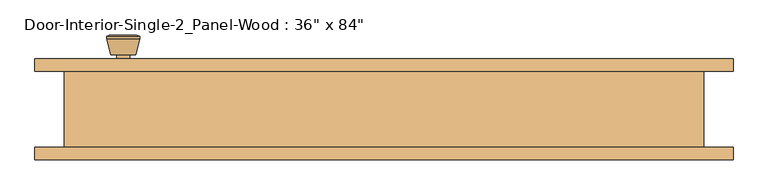
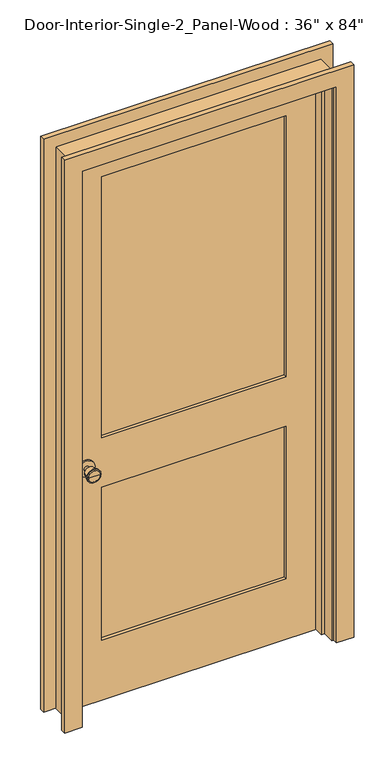
"""IFC4 building model written with IfcOpenShell, lengths in millimetres: door geometry."""

from ifc_helpers import new_model, si_unit, point, frame, frame_2d, origin, place, context, project, spatial, polyline, circle_curve, trimmed, segment, composite_curve, outline, extrude, faceted_brep, source, transform, mapped, element, save
from ifc_brep_helpers import plane_surface, cylinder_surface, revolved_surface, advanced_brep


def door_d4071c8b(model_context):
    return source(origin(), model_context, "Body", "SolidModel", [
        advanced_brep(
        [(-393.7, 13.05, 914.4), (-383.7, 13.05, 914.4), (-403.7, 13.05, 914.4), (-373.2241324, -35.95, 914.4), (-393.7, -35.95, 914.4), (-414.1758676, -35.95, 914.4), (-368.7, -34.1221319, 914.4), (-418.7, -34.1221319, 914.4), (-368.7, -30.6584537, 914.4), (-418.7, -30.6584537, 914.4), (-375.063764, -5.95, 914.4), (-412.336236, -5.95, 914.4), (-383.7, -5.95, 914.4), (-403.7, -5.95, 914.4)],
        [
            (0, 1),
            (1, 2, circle_curve(frame((-393.7, 13.05, 914.4), z_axis=(0.0, 1.0, 0.0), x_axis=(-1.0, 0.0, 0.0)), 10.0)),
            (2, 0),
            (2, 1, circle_curve(frame((-393.7, 13.05, 914.4), z_axis=(0.0, 1.0, 0.0), x_axis=(-1.0, 0.0, 0.0)), 10.0)),
            (3, 4),
            (4, 5),
            (5, 3, circle_curve(frame((-393.7, -35.95, 914.4), z_axis=(0.0, -1.0, 0.0), x_axis=(-1.0, 0.0, 0.0)), 20.4758676)),
            (3, 5, circle_curve(frame((-393.7, -35.95, 914.4), z_axis=(0.0, -1.0, 0.0), x_axis=(-1.0, 0.0, 0.0)), 20.4758676)),
            (6, 3),
            (5, 7),
            (7, 6, circle_curve(frame((-393.7, -34.1221319, 914.4), z_axis=(0.0, -1.0, 0.0), x_axis=(-1.0, 0.0, 0.0)), 25.0)),
            (6, 7, circle_curve(frame((-393.7, -34.1221319, 914.4), z_axis=(0.0, -1.0, 0.0), x_axis=(-1.0, 0.0, 0.0)), 25.0)),
            (8, 6),
            (7, 9),
            (9, 8, circle_curve(frame((-393.7, -30.6584537, 914.4), z_axis=(0.0, -1.0, 0.0), x_axis=(-1.0, 0.0, 0.0)), 25.0)),
            (8, 9, circle_curve(frame((-393.7, -30.6584537, 914.4), z_axis=(0.0, -1.0, 0.0), x_axis=(-1.0, 0.0, 0.0)), 25.0)),
            (10, 8),
            (9, 11),
            (11, 10, circle_curve(frame((-393.7, -5.95, 914.4), z_axis=(0.0, -1.0, 0.0), x_axis=(-1.0, 0.0, 0.0)), 18.636236)),
            (10, 11, circle_curve(frame((-393.7, -5.95, 914.4), z_axis=(0.0, -1.0, 0.0), x_axis=(-1.0, 0.0, 0.0)), 18.636236)),
            (12, 10),
            (11, 13),
            (13, 12, circle_curve(frame((-393.7, -5.95, 914.4), z_axis=(0.0, -1.0, 0.0), x_axis=(-1.0, 0.0, 0.0)), 10.0)),
            (12, 13, circle_curve(frame((-393.7, -5.95, 914.4), z_axis=(0.0, -1.0, 0.0), x_axis=(-1.0, 0.0, 0.0)), 10.0)),
            (1, 12),
            (13, 2),
        ],
        [
            plane_surface(frame((-393.7, 13.05, 914.4), z_axis=(0.0, 1.0, 0.0), x_axis=(-1.0, 0.0, 0.0))),
            plane_surface(frame((-393.7, -35.95, 914.4), z_axis=(0.0, -1.0, 0.0), x_axis=(-1.0, 0.0, 0.0))),
            revolved_surface(polyline([(-414.1758676, -35.95, 914.4), (-418.7, -34.1221319, 914.4)]), (-393.7, 13.05, 914.4), (0.0, 1.0, 0.0)),
            cylinder_surface(frame((-393.7, 13.05, 914.4), z_axis=(0.0, 1.0, 0.0), x_axis=(-1.0, 0.0, 0.0)), 25.0),
            revolved_surface(polyline([(-418.7, -30.6584537, 914.4), (-412.336236, -5.95, 914.4)]), (-393.7, 13.05, 914.4), (0.0, 1.0, 0.0)),
            plane_surface(frame((-393.7, -5.95, 914.4), z_axis=(0.0, 1.0, 0.0), x_axis=(-1.0, 0.0, 0.0))),
            cylinder_surface(frame((-393.7, 13.05, 914.4), z_axis=(0.0, 1.0, 0.0), x_axis=(-1.0, 0.0, 0.0)), 10.0),
        ],
        [
            (0, [[1, 2, 3]]),
            (0, [[-3, 4, -1]]),
            (1, [[5, 6, 7]]),
            (1, [[-6, -5, 8]]),
            (2, [[9, -7, 10, 11]]),
            (2, [[-10, -8, -9, 12]]),
            (3, [[13, -11, 14, 15]]),
            (3, [[-14, -12, -13, 16]]),
            (4, [[17, -15, 18, 19]]),
            (4, [[-18, -16, -17, 20]]),
            (5, [[21, -19, 22, 23]]),
            (5, [[-22, -20, -21, 24]]),
            (6, [[25, -23, 26, -2]]),
            (6, [[-26, -24, -25, -4]]),
        ],
    ),
        extrude(outline(composite_curve([segment(trimmed(circle_curve(frame_2d((914.4, -393.7)), 30.0), [point((914.4, -423.7))], [point((914.4, -363.7))], False, "CARTESIAN"), True, "CONTINUOUS"), segment(trimmed(circle_curve(frame_2d((914.4, -393.7)), 30.0), [point((914.4, -363.7))], [point((914.4, -423.7))], False, "CARTESIAN"), True, "CONTINUOUS")], self_intersect=False)), frame((0.0, 13.05, 0.0), z_axis=(0.0, 1.0, 0.0), x_axis=(0.0, 0.0, 1.0)), (0.0, 0.0, 1.0), 6.0),
        advanced_brep(
        [(-393.7, 59.975, 914.4), (-403.7, 59.975, 914.4), (-383.7, 59.975, 914.4), (-373.2241324, 108.975, 914.4), (-414.1758676, 108.975, 914.4), (-393.7, 108.975, 914.4), (-368.7, 107.1471319, 914.4), (-418.7, 107.1471319, 914.4), (-368.7, 103.6834537, 914.4), (-418.7, 103.6834537, 914.4), (-375.063764, 78.975, 914.4), (-412.336236, 78.975, 914.4), (-383.7, 78.975, 914.4), (-403.7, 78.975, 914.4)],
        [
            (0, 1),
            (1, 2, circle_curve(frame((-393.7, 59.975, 914.4), z_axis=(0.0, -1.0, 0.0), x_axis=(-1.0, 0.0, 0.0)), 10.0)),
            (2, 0),
            (2, 1, circle_curve(frame((-393.7, 59.975, 914.4), z_axis=(0.0, -1.0, 0.0), x_axis=(-1.0, 0.0, 0.0)), 10.0)),
            (3, 4, circle_curve(frame((-393.7, 108.975, 914.4), z_axis=(0.0, 1.0, 0.0), x_axis=(-1.0, 0.0, 0.0)), 20.4758676)),
            (4, 5),
            (5, 3),
            (4, 3, circle_curve(frame((-393.7, 108.975, 914.4), z_axis=(0.0, 1.0, 0.0), x_axis=(-1.0, 0.0, 0.0)), 20.4758676)),
            (6, 7, circle_curve(frame((-393.7, 107.1471319, 914.4), z_axis=(0.0, 1.0, 0.0), x_axis=(-1.0, 0.0, 0.0)), 25.0)),
            (7, 4),
            (3, 6),
            (7, 6, circle_curve(frame((-393.7, 107.1471319, 914.4), z_axis=(0.0, 1.0, 0.0), x_axis=(-1.0, 0.0, 0.0)), 25.0)),
            (8, 9, circle_curve(frame((-393.7, 103.6834537, 914.4), z_axis=(0.0, 1.0, 0.0), x_axis=(-1.0, 0.0, 0.0)), 25.0)),
            (9, 7),
            (6, 8),
            (9, 8, circle_curve(frame((-393.7, 103.6834537, 914.4), z_axis=(0.0, 1.0, 0.0), x_axis=(-1.0, 0.0, 0.0)), 25.0)),
            (10, 11, circle_curve(frame((-393.7, 78.975, 914.4), z_axis=(0.0, 1.0, 0.0), x_axis=(-1.0, 0.0, 0.0)), 18.636236)),
            (11, 9),
            (8, 10),
            (11, 10, circle_curve(frame((-393.7, 78.975, 914.4), z_axis=(0.0, 1.0, 0.0), x_axis=(-1.0, 0.0, 0.0)), 18.636236)),
            (12, 13, circle_curve(frame((-393.7, 78.975, 914.4), z_axis=(0.0, 1.0, 0.0), x_axis=(-1.0, 0.0, 0.0)), 10.0)),
            (13, 11),
            (10, 12),
            (13, 12, circle_curve(frame((-393.7, 78.975, 914.4), z_axis=(0.0, 1.0, 0.0), x_axis=(-1.0, 0.0, 0.0)), 10.0)),
            (1, 13),
            (12, 2),
        ],
        [
            plane_surface(frame((-393.7, 59.975, 914.4), z_axis=(0.0, -1.0, 0.0), x_axis=(-1.0, 0.0, 0.0))),
            plane_surface(frame((-393.7, 108.975, 914.4), z_axis=(0.0, 1.0, 0.0), x_axis=(-1.0, 0.0, 0.0))),
            revolved_surface(polyline([(-414.1758676, 108.975, 914.4), (-418.7, 107.1471319, 914.4)]), (-393.7, 59.975, 914.4), (0.0, -1.0, 0.0)),
            cylinder_surface(frame((-393.7, 59.975, 914.4), z_axis=(0.0, -1.0, 0.0), x_axis=(-1.0, 0.0, 0.0)), 25.0),
            revolved_surface(polyline([(-418.7, 103.6834537, 914.4), (-412.336236, 78.975, 914.4)]), (-393.7, 59.975, 914.4), (0.0, -1.0, 0.0)),
            plane_surface(frame((-393.7, 78.975, 914.4), z_axis=(0.0, -1.0, 0.0), x_axis=(-1.0, 0.0, 0.0))),
            cylinder_surface(frame((-393.7, 59.975, 914.4), z_axis=(0.0, -1.0, 0.0), x_axis=(-1.0, 0.0, 0.0)), 10.0),
        ],
        [
            (0, [[1, 2, 3]]),
            (0, [[-3, 4, -1]]),
            (1, [[5, 6, 7]]),
            (1, [[8, -7, -6]]),
            (2, [[9, 10, -5, 11]]),
            (2, [[12, -11, -8, -10]]),
            (3, [[13, 14, -9, 15]]),
            (3, [[16, -15, -12, -14]]),
            (4, [[17, 18, -13, 19]]),
            (4, [[20, -19, -16, -18]]),
            (5, [[21, 22, -17, 23]]),
            (5, [[24, -23, -20, -22]]),
            (6, [[-2, 25, -21, 26]]),
            (6, [[-4, -26, -24, -25]]),
        ],
    ),
        extrude(outline(composite_curve([segment(trimmed(circle_curve(frame_2d((914.4, -393.7)), 30.0), [point((914.4, -423.7))], [point((914.4, -363.7))], False, "CARTESIAN"), True, "CONTINUOUS"), segment(trimmed(circle_curve(frame_2d((914.4, -393.7)), 30.0), [point((914.4, -363.7))], [point((914.4, -423.7))], False, "CARTESIAN"), True, "CONTINUOUS")], self_intersect=False)), frame((0.0, 53.975, 0.0), z_axis=(0.0, 1.0, 0.0), x_axis=(0.0, 0.0, 1.0)), (0.0, 0.0, 1.0), 6.0),
        faceted_brep([(482.6, 53.975, 0.0), (482.6, -60.325, 0.0), (457.2, -60.325, 0.0), (457.2, -15.875, 0.0), (444.5, -15.875, 0.0), (444.5, 19.05, 0.0), (457.2, 19.05, 0.0), (457.2, 53.975, 0.0), (482.6, 53.975, 2159.0), (482.6, -60.325, 2159.0), (-482.6, -60.325, 2159.0), (-482.6, -60.325, 0.0), (-457.2, -60.325, 0.0), (-457.2, -60.325, 2133.6), (457.2, -60.325, 2133.6), (457.2, -15.875, 2133.6), (-457.2, -15.875, 2133.6), (-457.2, -15.875, 0.0), (-444.5, -15.875, 0.0), (-444.5, -15.875, 2120.9), (444.5, -15.875, 2120.9), (444.5, 19.05, 2120.9), (-444.5, 19.05, 2120.9), (-444.5, 19.05, 0.0), (-457.2, 19.05, 0.0), (-457.2, 19.05, 2133.6), (457.2, 19.05, 2133.6), (457.2, 53.975, 2133.6), (-457.2, 53.975, 2133.6), (-457.2, 53.975, 0.0), (-482.6, 53.975, 0.0), (-482.6, 53.975, 2159.0)], [[[0, 1, 2, 3, 4, 5, 6, 7]], [[1, 0, 8, 9]], [[2, 1, 9, 10, 11, 12, 13, 14]], [[3, 2, 14, 15]], [[4, 3, 15, 16, 17, 18, 19, 20]], [[5, 4, 20, 21]], [[6, 5, 21, 22, 23, 24, 25, 26]], [[7, 6, 26, 27]], [[0, 7, 27, 28, 29, 30, 31, 8]], [[9, 8, 31, 10]], [[15, 14, 13, 16]], [[21, 20, 19, 22]], [[27, 26, 25, 28]], [[30, 29, 24, 23, 18, 17, 12, 11]], [[10, 31, 30, 11]], [[16, 13, 12, 17]], [[22, 19, 18, 23]], [[28, 25, 24, 29]]]),
        extrude(outline(polyline([(2133.6, -457.2), (0.0, -457.2), (0.0, 457.2), (2133.6, 457.2), (2133.6, -457.2)]), holes=[polyline([(2014.5375, -336.55), (2014.5375, 336.55), (1009.65, 336.55), (1009.65, -336.55), (2014.5375, -336.55)]), polyline([(819.15, -336.55), (819.15, 336.55), (231.775, 336.55), (231.775, -336.55), (819.15, -336.55)])]), frame((0.0, 19.05, 0.0), z_axis=(0.0, 1.0, 0.0), x_axis=(0.0, 0.0, 1.0)), (0.0, 0.0, 1.0), 34.925),
        extrude(outline(polyline([(336.55, 30.6916667), (-336.55, 30.6916667), (-336.55, 42.3333333), (336.55, 42.3333333), (336.55, 30.6916667)])), frame((0.0, 0.0, 1009.65), z_axis=(0.0, 0.0, 1.0), x_axis=(1.0, 0.0, 0.0)), (0.0, 0.0, 1.0), 1004.8875),
        extrude(outline(polyline([(336.55, 30.6916667), (-336.55, 30.6916667), (-336.55, 42.3333333), (336.55, 42.3333333), (336.55, 30.6916667)])), frame((0.0, 0.0, 231.775), z_axis=(0.0, 0.0, 1.0), x_axis=(1.0, 0.0, 0.0)), (0.0, 0.0, 1.0), 587.375),
        extrude(outline(polyline([(0.0, 463.55), (0.0, 527.05), (2203.45, 527.05), (2203.45, -527.05), (0.0, -527.05), (0.0, -463.55), (2139.95, -463.55), (2139.95, 463.55), (0.0, 463.55)])), frame((0.0, 53.975, 0.0), z_axis=(0.0, 1.0, 0.0), x_axis=(0.0, 0.0, 1.0)), (0.0, 0.0, 1.0), 19.05),
        extrude(outline(polyline([(0.0, 463.55), (0.0, 527.05), (2203.45, 527.05), (2203.45, -527.05), (0.0, -527.05), (0.0, -463.55), (2139.95, -463.55), (2139.95, 463.55), (0.0, 463.55)])), frame((0.0, -79.375, 0.0), z_axis=(0.0, 1.0, 0.0), x_axis=(0.0, 0.0, 1.0)), (0.0, 0.0, 1.0), 19.05),
    ])


if __name__ == "__main__":
    model = new_model("IFC4")
    model_context = context("Model", 3, world=origin())
    ifc_project = project(units=[si_unit("LENGTHUNIT", "METRE", prefix="MILLI")], contexts=[model_context])
    site = spatial("IfcSite", under=ifc_project)
    building = spatial("IfcBuilding", under=site)
    placement = place(None, origin())
    door_shape = door_d4071c8b(model_context)
    element("IfcDoor", 1, ObjectType="Door-Interior-Single-2_Panel-Wood : 36\" x 84\"", at=placement, inside=building, context=model_context, shape_type="MappedRepresentation", body=[
        mapped(door_shape, transform((0.0, 0.0, 0.0), x_axis=(1.0, 0.0, 0.0), y_axis=(0.0, 1.0, 0.0), z_axis=(0.0, 0.0, 1.0))),
    ])
    save(model, "model.ifc")

# Revit data of these elements
# Type "Door-Interior-Single-2_Panel-Wood : 36\" x 84\""
#   Type Mark = "12"
#   Assembly Code = "C1020300"
#   Analytic Construction = "Wooden"
#   Top Rail = 0' - 4 11/16"
#   Thickness = 0' - 1 3/8"
#   Thermal Resistance (R) = 2.5876 (h·ft²·°F)/BTU
#   Swing Angle [instance default] = 90.00°
#   Stiles = 0' - 4 3/4"
#   Rough Width = 3' - 2"
#   Rough Height = 7' - 1"
#   Lock Rail = 0' - 7 1/2"
#   Height = 7' - 0"
#   Width = 3' - 0"
#   Heat Transfer Coefficient (U) = 0.3865 BTU/(h·ft²·°F)
#   Bottom Rail = 0' - 9 1/8"
#   Trim Material = Cherry
#   Panel Material = Cherry
#   Frame Material = Cherry
#   Door Handle Material = Aluminum
#   Visual Light Transmittance = 0
#   Solar Heat Gain Coefficient = 0
#   Wall Closure = (empty or 0)
#   Function = (empty or 0)
# Element 1 (IfcDoor, "Door-Interior-Single-2_Panel-Wood : 36\" x 84\"")
#   Materials on its faces: "Cherry", "Aluminum"
# Materials
#   "Cherry": class "Wood", colour RGB 226 177 128, transparency 0, Description = "Prunus Serotina", Cost = 0
#   "Aluminum": class "Metal", colour RGB 247 247 247, transparency 0, Description = "Aluminum 6061", Cost = 0
